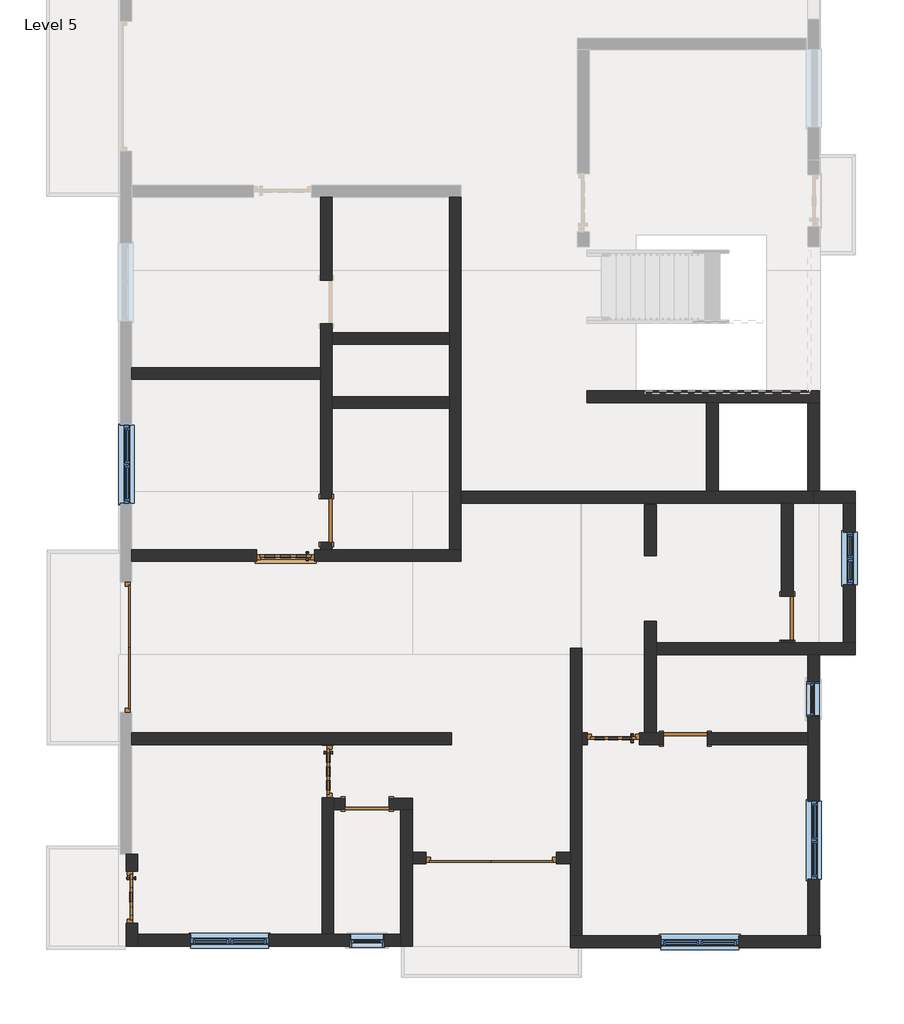
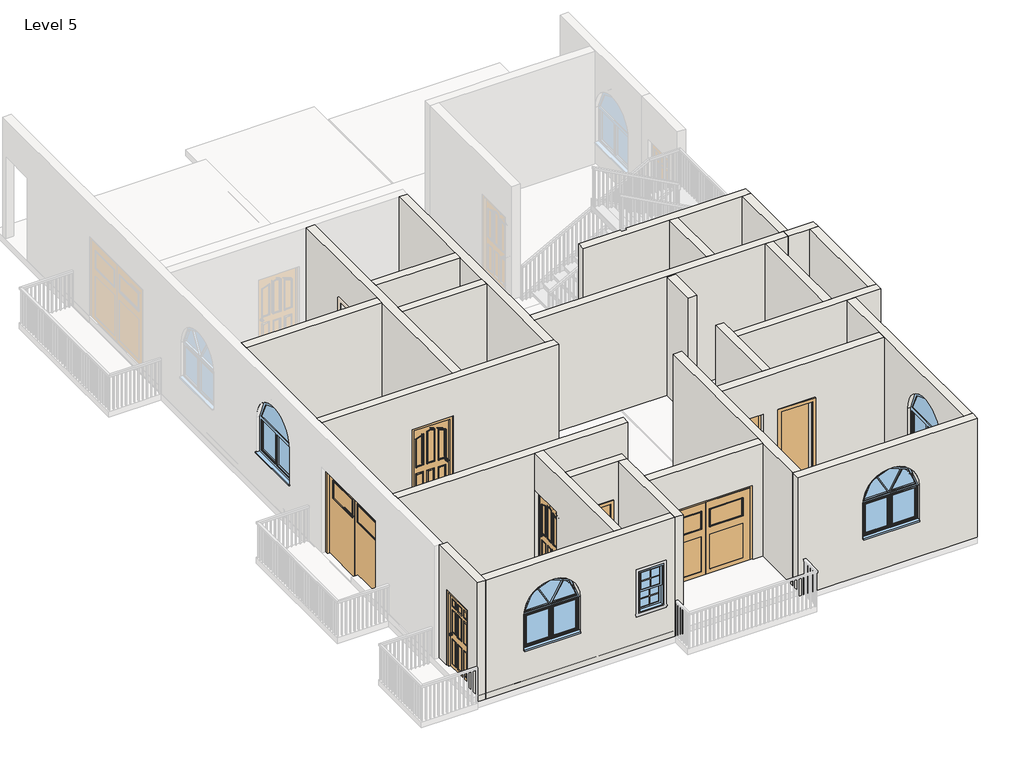
# One storey, part 1 of 7: 27 walls, 10 doors, 7 windows.
"""IFC4 building model written with IfcOpenShell, lengths in millimetres."""

from ifc_helpers import new_model, si_unit, frame, origin, place, context, project, spatial, polyline, circle_curve, outline, extrude, faceted_brep, transform, mapped, element, save
from ifc_brep_helpers import plane_surface, revolved_surface, advanced_brep
from components import doors_extsgl_5_910x2110mm_99758a98, doors_extsgl_6_1010x2110mm_b93c615f, doors_extsgl_6_1010x2110mm_efbaf1af, doors_extsgl_6_910x2110mm_72be2df1, doors_extsgl_6_910x2110mm_b26fcae4, doors_extsgl_6_910x2110mm_5dc58899, doors_extsgl_6_910x2110mm_16d7c084, doors_garage_timber_side_hung_glazing_2270x2050mm_ae99176d, doors_garage_timber_side_hung_glazing_2270x2200mm_badb7014, door_fadea3f2, door_53b1b562, window_679d2811, windows_arched_1360x910mm_c5754810, windows_dbl_w_glazing_bars_910x910mm_41eba874

model = new_model("IFC4")

# Units and contexts
model_context = context("Model", 3, world=origin())
ifc_project = project(units=[si_unit("LENGTHUNIT", "METRE", prefix="MILLI")], contexts=[model_context])

# Site, building, storey
site = spatial("IfcSite", under=ifc_project)
building = spatial("IfcBuilding", under=site)
storey = spatial("IfcBuildingStorey", under=building, Name="Level 5", Elevation=12192.0)

# Doors
placement = place(None, origin())
doors_extsgl_5_910x2110mm_shape = doors_extsgl_5_910x2110mm_99758a98(model_context)
element("IfcDoor", 1, ObjectType="Doors_ExtSgl_5 : 910x2110mm", at=placement, inside=storey, context=model_context, shape_type="MappedRepresentation", body=[
    mapped(doors_extsgl_5_910x2110mm_shape, transform((-6127.6013636, -9759.5108149, 12192.0), x_axis=(0.0, -1.0, 0.0), y_axis=(1.0, 0.0, 0.0), z_axis=(0.0, 0.0, 1.0))),
])
doors_extsgl_6_1010x2110mm_shape = doors_extsgl_6_1010x2110mm_b93c615f(model_context)
doors_extsgl_6_1010x2110mm_2_shape = doors_extsgl_6_1010x2110mm_efbaf1af(model_context)
element("IfcDoor", 2, ObjectType="Doors_ExtSgl_6 : 1010x2110mm", at=placement, inside=storey, context=model_context, shape_type="MappedRepresentation", body=[
    mapped(doors_extsgl_6_1010x2110mm_shape, transform((-3445.8775704, -3805.7037749, 12192.0), x_axis=(-1.0, 0.0, 0.0), y_axis=(0.0, -1.0, 0.0), z_axis=(0.0, 0.0, 1.0))),
    mapped(doors_extsgl_6_1010x2110mm_2_shape, transform((-3445.8775704, -3805.7037749, 12192.0), x_axis=(-1.0, 0.0, 0.0), y_axis=(0.0, -1.0, 0.0), z_axis=(0.0, 0.0, 1.0))),
])
doors_extsgl_6_910x2110mm_shape = doors_extsgl_6_910x2110mm_72be2df1(model_context)
doors_extsgl_6_910x2110mm_2_shape = doors_extsgl_6_910x2110mm_b26fcae4(model_context)
element("IfcDoor", 3, ObjectType="Doors_ExtSgl_6 : 910x2110mm", at=placement, inside=storey, context=model_context, shape_type="MappedRepresentation", body=[
    mapped(doors_extsgl_6_910x2110mm_shape, transform((2269.1224296, -6998.5466225, 12192.0), x_axis=(-1.0, 0.0, 0.0), y_axis=(0.0, -1.0, 0.0), z_axis=(0.0, 0.0, 1.0))),
    mapped(doors_extsgl_6_910x2110mm_2_shape, transform((2269.1224296, -6998.5466225, 12192.0), x_axis=(-1.0, 0.0, 0.0), y_axis=(0.0, -1.0, 0.0), z_axis=(0.0, 0.0, 1.0))),
])
doors_extsgl_6_910x2110mm_3_shape = doors_extsgl_6_910x2110mm_5dc58899(model_context)
doors_extsgl_6_910x2110mm_4_shape = doors_extsgl_6_910x2110mm_16d7c084(model_context)
element("IfcDoor", 4, ObjectType="Doors_ExtSgl_6 : 910x2110mm", at=placement, inside=storey, context=model_context, shape_type="MappedRepresentation", body=[
    mapped(doors_extsgl_6_910x2110mm_3_shape, transform((-2709.3109037, -7568.3747197, 12192.0), x_axis=(0.0, -1.0, 0.0), y_axis=(1.0, 0.0, 0.0), z_axis=(0.0, 0.0, 1.0))),
    mapped(doors_extsgl_6_910x2110mm_4_shape, transform((-2709.3109037, -7568.3747197, 12192.0), x_axis=(0.0, -1.0, 0.0), y_axis=(1.0, 0.0, 0.0), z_axis=(0.0, 0.0, 1.0))),
])
doors_garage_timber_side_hung_glazing_2270x2050mm_shape = doors_garage_timber_side_hung_glazing_2270x2050mm_ae99176d(model_context)
element("IfcDoor", 5, ObjectType="Doors_Garage_Timber_Side_Hung_Glazing : 2270x2050mm", at=placement, inside=storey, context=model_context, shape_type="MappedRepresentation", body=[
    mapped(doors_garage_timber_side_hung_glazing_2270x2050mm_shape, transform((141.8390963, -9078.0694836, 12192.0), x_axis=(-1.0, 0.0, 0.0), y_axis=(0.0, -1.0, 0.0), z_axis=(0.0, 0.0, 1.0))),
])
doors_garage_timber_side_hung_glazing_2270x2200mm_shape = doors_garage_timber_side_hung_glazing_2270x2200mm_badb7014(model_context)
element("IfcDoor", 6, ObjectType="Doors_Garage_Timber_Side_Hung_Glazing : 2270x2200mm", at=placement, inside=storey, context=model_context, shape_type="MappedRepresentation", body=[
    mapped(doors_garage_timber_side_hung_glazing_2270x2200mm_shape, transform((-6229.2013636, -5402.1251987, 12192.0), x_axis=(0.0, 1.0, 0.0), y_axis=(-1.0, 0.0, 0.0), z_axis=(0.0, 0.0, 1.0))),
])
door_shape = door_fadea3f2(model_context)
element("IfcDoor", 7, ObjectType="Single-Flush : 30\" x 80\"", at=placement, inside=storey, context=model_context, shape_type="MappedRepresentation", body=[
    mapped(door_shape, transform((-2023.5109037, -8138.2694836, 12192.0), x_axis=(-1.0, 0.0, 0.0), y_axis=(0.0, -1.0, 0.0), z_axis=(0.0, 0.0, 1.0))),
])
element("IfcDoor", 8, ObjectType="Single-Flush : 30\" x 80\"", at=placement, inside=storey, context=model_context, shape_type="MappedRepresentation", body=[
    mapped(door_shape, transform((5304.3890963, -4897.9037749, 12192.0), x_axis=(0.0, -1.0, 0.0), y_axis=(1.0, 0.0, 0.0), z_axis=(0.0, 0.0, 1.0))),
])
door_2_shape = door_53b1b562(model_context)
element("IfcDoor", 9, ObjectType="Single-Flush : 30\" x 80\"", at=placement, inside=storey, context=model_context, shape_type="MappedRepresentation", body=[
    mapped(door_2_shape, transform((-2734.7109037, -3196.1037749, 12192.0), x_axis=(0.0, 1.0, 0.0), y_axis=(-1.0, 0.0, 0.0), z_axis=(0.0, 0.0, 1.0))),
])
element("IfcDoor", 10, ObjectType="Single-Flush : 30\" x 80\"", at=placement, inside=storey, context=model_context, shape_type="MappedRepresentation", body=[
    mapped(door_2_shape, transform((3526.3890963, -6998.5466225, 12192.0), x_axis=(-1.0, 0.0, 0.0), y_axis=(0.0, -1.0, 0.0), z_axis=(0.0, 0.0, 1.0))),
])

# Walls
element("IfcWall", 11, ObjectType="Generic - 9\" w", at=placement, inside=storey, context=model_context, shape_type="Brep", body=[
    faceted_brep([(6485.4890963, -2688.1037749, 12192.0), (5863.1890963, -2688.1037749, 12192.0), (5761.5890963, -2688.1037749, 12192.0), (5761.5890963, -2688.1037749, 15240.0), (5863.1890963, -2688.1037749, 15240.0), (6485.4890963, -2688.1037749, 15240.0), (6485.4890963, -2891.3037749, 12192.0), (6485.4890963, -2891.3037749, 15240.0), (6282.2890963, -2891.3037749, 15240.0), (5761.5890963, -2891.3037749, 15240.0), (5761.5890963, -2891.3037749, 12192.0), (6282.2890963, -2891.3037749, 12192.0)], [[[0, 1, 2, 3, 4, 5]], [[6, 7, 8, 9, 10, 11]], [[2, 1, 0, 6, 11, 10]], [[3, 2, 10, 9]], [[5, 4, 3, 9, 8, 7]], [[0, 5, 7, 6]]]),
])
element("IfcWall", 12, ObjectType="Generic - 9\" w", at=placement, inside=storey, context=model_context, shape_type="Brep", body=[
    faceted_brep([(5761.5890963, -2688.1037749, 12192.0), (5659.9890963, -2688.1037749, 12192.0), (4097.8890963, -2688.1037749, 12192.0), (3894.6890963, -2688.1037749, 12192.0), (-385.2109037, -2688.1037749, 12192.0), (-385.2109037, -2688.1037749, 15240.0), (3894.6890963, -2688.1037749, 15240.0), (4097.8890963, -2688.1037749, 15240.0), (5659.9890963, -2688.1037749, 15240.0), (5761.5890963, -2688.1037749, 15240.0), (5761.5890963, -2891.3037749, 12192.0), (5761.5890963, -2891.3037749, 15240.0), (5405.9890963, -2891.3037749, 15240.0), (5202.7890963, -2891.3037749, 15240.0), (-385.2109037, -2891.3037749, 15240.0), (-385.2109037, -2891.3037749, 12192.0), (5202.7890963, -2891.3037749, 12192.0), (5405.9890963, -2891.3037749, 12192.0)], [[[0, 1, 2, 3, 4, 5, 6, 7, 8, 9]], [[10, 11, 12, 13, 14, 15, 16, 17]], [[4, 3, 2, 1, 0, 10, 17, 16, 15]], [[9, 8, 7, 6, 5, 14, 13, 12, 11]], [[0, 9, 11, 10]], [[5, 4, 15, 14]]]),
])
element("IfcWall", 13, ObjectType="Generic - 9\" w", at=placement, inside=storey, context=model_context, shape_type="SweptSolid", body=[
    extrude(outline(polyline([(3894.6890963, -2688.1037749), (3894.6890963, -1138.7037749), (4097.8890963, -1138.7037749), (4097.8890963, -2688.1037749), (3894.6890963, -2688.1037749)])), frame((0.0, 0.0, 12192.0), z_axis=(0.0, 0.0, 1.0), x_axis=(1.0, 0.0, 0.0)), (0.0, 0.0, 1.0), 3048.0),
])
element("IfcWall", 14, ObjectType="Generic - 9\" w", at=placement, inside=storey, context=model_context, shape_type="Brep", body=[
    faceted_brep([(5863.1890963, -935.5037749, 12192.0), (1812.4805171, -935.5037749, 12192.0), (1812.4805171, -935.5037749, 15240.0), (5863.1890963, -935.5037749, 15240.0), (5863.1890963, -1138.7037749, 12192.0), (5863.1890963, -1138.7037749, 15240.0), (5659.9890963, -1138.7037749, 15240.0), (4097.8890963, -1138.7037749, 15240.0), (3894.6890963, -1138.7037749, 15240.0), (1812.4805171, -1138.7037749, 15240.0), (1812.4805171, -1138.7037749, 12192.0), (3894.6890963, -1138.7037749, 12192.0), (4097.8890963, -1138.7037749, 12192.0), (5659.9890963, -1138.7037749, 12192.0)], [[[0, 1, 2, 3]], [[4, 5, 6, 7, 8, 9, 10, 11, 12, 13]], [[1, 0, 4, 13, 12, 11, 10]], [[2, 1, 10, 9]], [[3, 2, 9, 8, 7, 6, 5]], [[0, 3, 5, 4]]]),
])
element("IfcWall", 15, ObjectType="Generic - 9\" w", at=placement, inside=storey, context=model_context, shape_type="AdvancedBrep", body=[
    advanced_brep(
    [(1519.7890963, -10638.3037749, 12192.0), (5875.8890963, -10638.3037749, 12192.0), (5875.8890963, -10638.3037749, 15240.0), (1519.7890963, -10638.3037749, 15240.0), (4460.3890963, -10638.3037749, 13106.4), (3100.3890963, -10638.3037749, 13106.4), (3100.3890963, -10638.3037749, 14016.4), (4460.3890963, -10638.3037749, 14016.4), (1519.7890963, -10435.1037749, 12192.0), (1519.7890963, -10435.1037749, 15240.0), (1722.9890963, -10435.1037749, 15240.0), (5659.9890963, -10435.1037749, 15240.0), (5863.1890963, -10435.1037749, 15240.0), (5875.8890963, -10435.1037749, 15240.0), (5875.8890963, -10435.1037749, 12192.0), (5863.1890963, -10435.1037749, 12192.0), (5659.9890963, -10435.1037749, 12192.0), (1722.9890963, -10435.1037749, 12192.0), (4460.3890963, -10435.1037749, 13106.4), (4460.3890963, -10435.1037749, 14016.4), (3100.3890963, -10435.1037749, 14016.4), (3100.3890963, -10435.1037749, 13106.4)],
    [
        (0, 1),
        (1, 2),
        (2, 3),
        (3, 0),
        (4, 5),
        (5, 6),
        (6, 7, circle_curve(frame((3780.3890963, -10638.3037749, 14016.4), z_axis=(0.0, 1.0, 0.0), x_axis=(-1.0, 0.0, 0.0)), 680.0)),
        (7, 4),
        (8, 9),
        (9, 10),
        (10, 11),
        (11, 12),
        (12, 13),
        (13, 14),
        (14, 15),
        (15, 16),
        (16, 17),
        (17, 8),
        (18, 19),
        (19, 20, circle_curve(frame((3780.3890963, -10435.1037749, 14016.4), z_axis=(0.0, -1.0, 0.0), x_axis=(-1.0, 0.0, 0.0)), 680.0)),
        (20, 21),
        (21, 18),
        (0, 8),
        (14, 1),
        (13, 2),
        (9, 3),
        (18, 4),
        (7, 19),
        (6, 20),
        (5, 21),
    ],
    [
        plane_surface(frame((1722.9890963, -10638.3037749, 12192.0), z_axis=(0.0, -1.0, 0.0), x_axis=(1.0, 0.0, 0.0))),
        plane_surface(frame((1722.9890963, -10435.1037749, 12192.0), z_axis=(0.0, 1.0, 0.0), x_axis=(-1.0, 0.0, 0.0))),
        plane_surface(frame((1621.3890963, -10638.3037749, 12192.0), z_axis=(0.0, 0.0, -1.0), x_axis=(0.0, 1.0, 0.0))),
        plane_surface(frame((5875.8890963, -10638.3037749, 12192.0), z_axis=(1.0, 0.0, 0.0), x_axis=(0.0, 1.0, 0.0))),
        plane_surface(frame((5875.8890963, -10638.3037749, 15240.0), z_axis=(0.0, 0.0, 1.0), x_axis=(0.0, 1.0, 0.0))),
        plane_surface(frame((1519.7890963, -5418.6037749, 12192.0), z_axis=(-1.0, 0.0, 0.0), x_axis=(0.0, -1.0, 0.0))),
        plane_surface(frame((4460.3890963, -10435.1037749, 13106.4), z_axis=(-1.0, 0.0, 0.0), x_axis=(0.0, -1.0, 0.0))),
        revolved_surface(polyline([(3100.3890963, -10638.3037749, 14016.4), (3100.3890963, -10435.1037749, 14016.4)]), (3780.3890963, -10435.1037749, 14016.4), (0.0, -1.0, 0.0)),
        plane_surface(frame((3100.3890963, -10435.1037749, 14016.4), z_axis=(1.0, 0.0, 0.0), x_axis=(0.0, -1.0, 0.0))),
        plane_surface(frame((3100.3890963, -10435.1037749, 13106.4), z_axis=(0.0, 0.0, 1.0), x_axis=(0.0, -1.0, 0.0))),
    ],
    [
        (0, [[1, 2, 3, 4], [5, 6, 7, 8]]),
        (1, [[9, 10, 11, 12, 13, 14, 15, 16, 17, 18], [19, 20, 21, 22]]),
        (2, [[-1, 23, -18, -17, -16, -15, 24]]),
        (3, [[-2, -24, -14, 25]]),
        (4, [[-3, -25, -13, -12, -11, -10, 26]]),
        (5, [[-4, -26, -9, -23]]),
        (6, [[-19, 27, -8, 28]]),
        (7, [[-20, -28, -7, 29]]),
        (8, [[-21, -29, -6, 30]]),
        (9, [[-22, -30, -5, -27]]),
    ],
),
])
element("IfcWall", 16, ObjectType="Generic - 9\" w", at=placement, inside=storey, context=model_context, shape_type="AdvancedBrep", body=[
    advanced_brep(
    [(5863.1890963, -10435.1037749, 12192.0), (5863.1890963, -5532.9037749, 12192.0), (5863.1890963, -5532.9037749, 15240.0), (5863.1890963, -10435.1037749, 15240.0), (5863.1890963, -8087.6251987, 13106.4), (5863.1890963, -9447.6251987, 13106.4), (5863.1890963, -9447.6251987, 14016.4), (5863.1890963, -8087.6251987, 14016.4), (5863.1890963, -6618.7537749, 14173.2), (5863.1890963, -6009.1537749, 14173.2), (5863.1890963, -6009.1537749, 13106.4), (5863.1890963, -6618.7537749, 13106.4), (5659.9890963, -10435.1037749, 12192.0), (5659.9890963, -10435.1037749, 15240.0), (5659.9890963, -7100.1466225, 15240.0), (5659.9890963, -6896.9466225, 15240.0), (5659.9890963, -5532.9037749, 15240.0), (5659.9890963, -5532.9037749, 12192.0), (5659.9890963, -6896.9466225, 12192.0), (5659.9890963, -7100.1466225, 12192.0), (5659.9890963, -8087.6251987, 13106.4), (5659.9890963, -8087.6251987, 14016.4), (5659.9890963, -9447.6251987, 14016.4), (5659.9890963, -9447.6251987, 13106.4), (5659.9890963, -6618.7537749, 14173.2), (5659.9890963, -6618.7537749, 13106.4), (5659.9890963, -6009.1537749, 13106.4), (5659.9890963, -6009.1537749, 14173.2)],
    [
        (0, 1),
        (1, 2),
        (2, 3),
        (3, 0),
        (4, 5),
        (5, 6),
        (6, 7, circle_curve(frame((5863.1890963, -8767.6251987, 14016.4), z_axis=(-1.0, 0.0, 0.0), x_axis=(0.0, -1.0, 0.0)), 680.0)),
        (7, 4),
        (8, 9),
        (9, 10),
        (10, 11),
        (11, 8),
        (12, 13),
        (13, 14),
        (14, 15),
        (15, 16),
        (16, 17),
        (17, 18),
        (18, 19),
        (19, 12),
        (20, 21),
        (21, 22, circle_curve(frame((5659.9890963, -8767.6251987, 14016.4), z_axis=(1.0, 0.0, 0.0), x_axis=(0.0, -1.0, 0.0)), 680.0)),
        (22, 23),
        (23, 20),
        (24, 25),
        (25, 26),
        (26, 27),
        (27, 24),
        (0, 12),
        (17, 1),
        (2, 16),
        (13, 3),
        (20, 4),
        (7, 21),
        (6, 22),
        (5, 23),
        (24, 8),
        (11, 25),
        (10, 26),
        (9, 27),
    ],
    [
        plane_surface(frame((5863.1890963, -10435.1037749, 12192.0), z_axis=(1.0, 0.0, 0.0), x_axis=(0.0, 1.0, 0.0))),
        plane_surface(frame((5659.9890963, -10435.1037749, 12192.0), z_axis=(-1.0, 0.0, 0.0), x_axis=(0.0, -1.0, 0.0))),
        plane_surface(frame((5863.1890963, -10536.7037749, 12192.0), z_axis=(0.0, 0.0, -1.0), x_axis=(-1.0, 0.0, 0.0))),
        plane_surface(frame((5863.1890963, -5431.3037749, 15240.0), z_axis=(0.0, 0.0, 1.0), x_axis=(-1.0, 0.0, 0.0))),
        plane_surface(frame((1722.9890963, -10435.1037749, 12192.0), z_axis=(0.0, -1.0, 0.0), x_axis=(-1.0, 0.0, 0.0))),
        plane_surface(frame((3018.3890963, -5532.9037749, 12192.0), z_axis=(0.0, 1.0, 0.0), x_axis=(1.0, 0.0, 0.0))),
        plane_surface(frame((5659.9890963, -8087.6251987, 13106.4), z_axis=(0.0, -1.0, 0.0), x_axis=(1.0, 0.0, 0.0))),
        revolved_surface(polyline([(5863.1890963, -9447.6251987, 14016.4), (5659.9890963, -9447.6251987, 14016.4)]), (5659.9890963, -8767.6251987, 14016.4), (1.0, 0.0, 0.0)),
        plane_surface(frame((5659.9890963, -9447.6251987, 14016.4), z_axis=(0.0, 1.0, 0.0), x_axis=(1.0, 0.0, 0.0))),
        plane_surface(frame((5659.9890963, -9447.6251987, 13106.4), z_axis=(0.0, 0.0, 1.0), x_axis=(1.0, 0.0, 0.0))),
        plane_surface(frame((5659.9890963, -6618.7537749, 14173.2), z_axis=(0.0, 1.0, 0.0), x_axis=(1.0, 0.0, 0.0))),
        plane_surface(frame((5659.9890963, -6618.7537749, 13106.4), z_axis=(0.0, 0.0, 1.0), x_axis=(1.0, 0.0, 0.0))),
        plane_surface(frame((5659.9890963, -6009.1537749, 13106.4), z_axis=(0.0, -1.0, 0.0), x_axis=(1.0, 0.0, 0.0))),
        plane_surface(frame((5659.9890963, -6009.1537749, 14173.2), z_axis=(0.0, 0.0, -1.0), x_axis=(1.0, 0.0, 0.0))),
    ],
    [
        (0, [[1, 2, 3, 4], [5, 6, 7, 8], [9, 10, 11, 12]]),
        (1, [[13, 14, 15, 16, 17, 18, 19, 20], [21, 22, 23, 24], [25, 26, 27, 28]]),
        (2, [[-1, 29, -20, -19, -18, 30]]),
        (3, [[-3, 31, -16, -15, -14, 32]]),
        (4, [[-4, -32, -13, -29]]),
        (5, [[-2, -30, -17, -31]]),
        (6, [[-21, 33, -8, 34]]),
        (7, [[-22, -34, -7, 35]]),
        (8, [[-23, -35, -6, 36]]),
        (9, [[-24, -36, -5, -33]]),
        (10, [[-25, 37, -12, 38]]),
        (11, [[-26, -38, -11, 39]]),
        (12, [[-27, -39, -10, 40]]),
        (13, [[-28, -40, -9, -37]]),
    ],
),
])
element("IfcWall", 17, ObjectType="Generic - 9\" w", at=placement, inside=storey, context=model_context, shape_type="Brep", body=[
    faceted_brep([(5659.9890963, -1138.7037749, 12192.0), (5659.9890963, -2688.1037749, 12192.0), (5659.9890963, -2688.1037749, 15240.0), (5659.9890963, -1138.7037749, 15240.0), (5863.1890963, -1138.7037749, 12192.0), (5863.1890963, -1138.7037749, 15240.0), (5863.1890963, -2688.1037749, 15240.0), (5863.1890963, -2688.1037749, 12192.0), (5761.5890963, -2688.1037749, 12192.0), (5761.5890963, -2688.1037749, 15240.0)], [[[0, 1, 2, 3]], [[4, 5, 6, 7]], [[1, 0, 4, 7, 8]], [[3, 2, 9, 6, 5]], [[2, 1, 8, 7, 6, 9]], [[0, 3, 5, 4]]]),
])
element("IfcWall", 18, ObjectType="Generic - 9\" w", at=placement, inside=storey, context=model_context, shape_type="Brep", body=[
    faceted_brep([(-6229.2013636, -10214.5441482, 14302.0), (-6229.2013636, -10214.5441482, 12192.0), (-6229.2013636, -10612.9037749, 12192.0), (-6229.2013636, -10612.9037749, 15240.0), (-6229.2013636, -9007.7845215, 15240.0), (-6229.2013636, -9007.7845215, 12192.0), (-6229.2013636, -9304.5441482, 12192.0), (-6229.2013636, -9304.5441482, 14302.0), (-6026.0013636, -10612.9037749, 12192.0), (-6026.0013636, -10409.7037749, 12192.0), (-6026.0013636, -10214.5441482, 12192.0), (-6026.0013636, -10214.5441482, 14302.0), (-6026.0013636, -9304.5441482, 14302.0), (-6026.0013636, -9304.5441482, 12192.0), (-6026.0013636, -9007.7845215, 12192.0), (-6026.0013636, -9007.7845215, 15240.0), (-6026.0013636, -10409.7037749, 15240.0), (-6026.0013636, -10612.9037749, 15240.0), (-6127.6013636, -9007.7845215, 12192.0), (-6127.6013636, -9007.7845215, 15240.0)], [[[0, 1, 2, 3, 4, 5, 6, 7]], [[8, 9, 10, 11, 12, 13, 14, 15, 16, 17]], [[6, 5, 18, 14, 13]], [[2, 1, 10, 9, 8]], [[4, 3, 17, 16, 15, 19]], [[5, 4, 19, 15, 14, 18]], [[13, 12, 7, 6]], [[11, 10, 1, 0]], [[12, 11, 0, 7]], [[3, 2, 8, 17]]]),
])
element("IfcWall", 19, ObjectType="Generic - 9\" w", at=placement, inside=storey, context=model_context, shape_type="AdvancedBrep", body=[
    advanced_brep(
    [(-6026.0013636, -10612.9037749, 12192.0), (-1439.3109037, -10612.9037749, 12192.0), (-1439.3109037, -10612.9037749, 15240.0), (-6026.0013636, -10612.9037749, 15240.0), (-3738.4561337, -10612.9037749, 13106.4), (-5098.4561337, -10612.9037749, 13106.4), (-5098.4561337, -10612.9037749, 14016.4), (-3738.4561337, -10612.9037749, 14016.4), (-1718.7109037, -10612.9037749, 14173.2), (-1718.7109037, -10612.9037749, 13106.4), (-2328.3109037, -10612.9037749, 13106.4), (-2328.3109037, -10612.9037749, 14173.2), (-6026.0013636, -10409.7037749, 12192.0), (-6026.0013636, -10409.7037749, 15240.0), (-2810.9109037, -10409.7037749, 15240.0), (-2607.7109037, -10409.7037749, 15240.0), (-1439.3109037, -10409.7037749, 15240.0), (-1439.3109037, -10409.7037749, 12192.0), (-2607.7109037, -10409.7037749, 12192.0), (-2810.9109037, -10409.7037749, 12192.0), (-3738.4561337, -10409.7037749, 13106.4), (-3738.4561337, -10409.7037749, 14016.4), (-5098.4561337, -10409.7037749, 14016.4), (-5098.4561337, -10409.7037749, 13106.4), (-1718.7109037, -10409.7037749, 14173.2), (-2328.3109037, -10409.7037749, 14173.2), (-2328.3109037, -10409.7037749, 13106.4), (-1718.7109037, -10409.7037749, 13106.4)],
    [
        (0, 1),
        (1, 2),
        (2, 3),
        (3, 0),
        (4, 5),
        (5, 6),
        (6, 7, circle_curve(frame((-4418.4561337, -10612.9037749, 14016.4), z_axis=(0.0, 1.0, 0.0), x_axis=(-1.0, 0.0, 0.0)), 680.0)),
        (7, 4),
        (8, 9),
        (9, 10),
        (10, 11),
        (11, 8),
        (12, 13),
        (13, 14),
        (14, 15),
        (15, 16),
        (16, 17),
        (17, 18),
        (18, 19),
        (19, 12),
        (20, 21),
        (21, 22, circle_curve(frame((-4418.4561337, -10409.7037749, 14016.4), z_axis=(0.0, -1.0, 0.0), x_axis=(-1.0, 0.0, 0.0)), 680.0)),
        (22, 23),
        (23, 20),
        (24, 25),
        (25, 26),
        (26, 27),
        (27, 24),
        (0, 12),
        (17, 1),
        (2, 16),
        (13, 3),
        (20, 4),
        (7, 21),
        (6, 22),
        (5, 23),
        (8, 24),
        (27, 9),
        (26, 10),
        (25, 11),
    ],
    [
        plane_surface(frame((-6229.2013636, -10612.9037749, 12192.0), z_axis=(0.0, -1.0, 0.0), x_axis=(1.0, 0.0, 0.0))),
        plane_surface(frame((-6229.2013636, -10409.7037749, 12192.0), z_axis=(0.0, 1.0, 0.0), x_axis=(-1.0, 0.0, 0.0))),
        plane_surface(frame((-6127.6013636, -10612.9037749, 12192.0), z_axis=(0.0, 0.0, -1.0), x_axis=(0.0, 1.0, 0.0))),
        plane_surface(frame((-1337.7109037, -10612.9037749, 15240.0), z_axis=(0.0, 0.0, 1.0), x_axis=(0.0, 1.0, 0.0))),
        plane_surface(frame((-1439.3109037, -8239.8694836, 12192.0), z_axis=(1.0, 0.0, 0.0), x_axis=(0.0, -1.0, 0.0))),
        plane_surface(frame((-6026.0013636, -9109.3845215, 12192.0), z_axis=(-1.0, 0.0, 0.0), x_axis=(0.0, 1.0, 0.0))),
        plane_surface(frame((-3738.4561337, -10409.7037749, 13106.4), z_axis=(-1.0, 0.0, 0.0), x_axis=(0.0, -1.0, 0.0))),
        revolved_surface(polyline([(-5098.4561337, -10612.9037749, 14016.4), (-5098.4561337, -10409.7037749, 14016.4)]), (-4418.4561337, -10409.7037749, 14016.4), (0.0, -1.0, 0.0)),
        plane_surface(frame((-5098.4561337, -10409.7037749, 14016.4), z_axis=(1.0, 0.0, 0.0), x_axis=(0.0, -1.0, 0.0))),
        plane_surface(frame((-5098.4561337, -10409.7037749, 13106.4), z_axis=(0.0, 0.0, 1.0), x_axis=(0.0, -1.0, 0.0))),
        plane_surface(frame((-1718.7109037, -10612.9037749, 14173.2), z_axis=(-1.0, 0.0, 0.0), x_axis=(0.0, 1.0, 0.0))),
        plane_surface(frame((-1718.7109037, -10612.9037749, 13106.4), z_axis=(0.0, 0.0, 1.0), x_axis=(0.0, 1.0, 0.0))),
        plane_surface(frame((-2328.3109037, -10612.9037749, 13106.4), z_axis=(1.0, 0.0, 0.0), x_axis=(0.0, 1.0, 0.0))),
        plane_surface(frame((-2328.3109037, -10612.9037749, 14173.2), z_axis=(0.0, 0.0, -1.0), x_axis=(0.0, 1.0, 0.0))),
    ],
    [
        (0, [[1, 2, 3, 4], [5, 6, 7, 8], [9, 10, 11, 12]]),
        (1, [[13, 14, 15, 16, 17, 18, 19, 20], [21, 22, 23, 24], [25, 26, 27, 28]]),
        (2, [[-1, 29, -20, -19, -18, 30]]),
        (3, [[-3, 31, -16, -15, -14, 32]]),
        (4, [[-2, -30, -17, -31]]),
        (5, [[-4, -32, -13, -29]]),
        (6, [[-21, 33, -8, 34]]),
        (7, [[-22, -34, -7, 35]]),
        (8, [[-23, -35, -6, 36]]),
        (9, [[-24, -36, -5, -33]]),
        (10, [[-9, 37, -28, 38]]),
        (11, [[-10, -38, -27, 39]]),
        (12, [[-11, -39, -26, 40]]),
        (13, [[-12, -40, -25, -37]]),
    ],
),
])
element("IfcWall", 20, ObjectType="Generic -4.5\" p", at=placement, inside=storey, context=model_context, shape_type="Brep", body=[
    faceted_brep([(-2836.3109037, 232.8962251, 12192.0), (-2836.3109037, -529.1037749, 12192.0), (-2836.3109037, -732.3037749, 12192.0), (-2836.3109037, -2815.1037749, 12192.0), (-2836.3109037, -2815.1037749, 14224.0), (-2836.3109037, -3577.1037749, 14224.0), (-2836.3109037, -3577.1037749, 12192.0), (-2836.3109037, -3704.1037749, 12192.0), (-2836.3109037, -3704.1037749, 15240.0), (-2836.3109037, -732.3037749, 15240.0), (-2836.3109037, -529.1037749, 15240.0), (-2836.3109037, 2442.6962251, 15240.0), (-2836.3109037, 2442.6962251, 12192.0), (-2836.3109037, 994.8962251, 12192.0), (-2836.3109037, 994.8962251, 14224.0), (-2836.3109037, 232.8962251, 14224.0), (-2633.1109037, -2815.1037749, 14224.0), (-2633.1109037, -2815.1037749, 12192.0), (-2633.1109037, -1240.3037749, 12192.0), (-2633.1109037, -1037.1037749, 12192.0), (-2633.1109037, -122.7037749, 12192.0), (-2633.1109037, 80.4962251, 12192.0), (-2633.1109037, 232.8962251, 12192.0), (-2633.1109037, 232.8962251, 14224.0), (-2633.1109037, 994.8962251, 14224.0), (-2633.1109037, 994.8962251, 12192.0), (-2633.1109037, 2442.6962251, 12192.0), (-2633.1109037, 2442.6962251, 15240.0), (-2633.1109037, 80.4962251, 15240.0), (-2633.1109037, -122.7037749, 15240.0), (-2633.1109037, -1037.1037749, 15240.0), (-2633.1109037, -1240.3037749, 15240.0), (-2633.1109037, -3704.1037749, 15240.0), (-2633.1109037, -3704.1037749, 12192.0), (-2633.1109037, -3577.1037749, 12192.0), (-2633.1109037, -3577.1037749, 14224.0)], [[[0, 1, 2, 3, 4, 5, 6, 7, 8, 9, 10, 11, 12, 13, 14, 15]], [[16, 17, 18, 19, 20, 21, 22, 23, 24, 25, 26, 27, 28, 29, 30, 31, 32, 33, 34, 35]], [[26, 25, 13, 12]], [[34, 33, 7, 6]], [[22, 21, 20, 19, 18, 17, 3, 2, 1, 0]], [[11, 10, 9, 8, 32, 31, 30, 29, 28, 27]], [[12, 11, 27, 26]], [[8, 7, 33, 32]], [[14, 13, 25, 24]], [[15, 14, 24, 23]], [[0, 15, 23, 22]], [[4, 3, 17, 16]], [[5, 4, 16, 35]], [[6, 5, 35, 34]]]),
])
element("IfcWall", 21, ObjectType="Generic -4.5\" p", at=placement, inside=storey, context=model_context, shape_type="Brep", body=[
    faceted_brep([(-6127.6013636, -3907.3037749, 12192.0), (-3950.9109037, -3907.3037749, 12192.0), (-3950.9109037, -3907.3037749, 14302.0), (-2940.9109037, -3907.3037749, 14302.0), (-2940.9109037, -3907.3037749, 12192.0), (-385.2109037, -3907.3037749, 12192.0), (-385.2109037, -3907.3037749, 15240.0), (-6127.6013636, -3907.3037749, 15240.0), (-3950.9109037, -3704.1037749, 14302.0), (-3950.9109037, -3704.1037749, 12192.0), (-6127.6013636, -3704.1037749, 12192.0), (-6127.6013636, -3704.1037749, 15240.0), (-2836.3109037, -3704.1037749, 15240.0), (-2633.1109037, -3704.1037749, 15240.0), (-588.4109037, -3704.1037749, 15240.0), (-385.2109037, -3704.1037749, 15240.0), (-385.2109037, -3704.1037749, 12192.0), (-588.4109037, -3704.1037749, 12192.0), (-2633.1109037, -3704.1037749, 12192.0), (-2836.3109037, -3704.1037749, 12192.0), (-2940.9109037, -3704.1037749, 12192.0), (-2940.9109037, -3704.1037749, 14302.0)], [[[0, 1, 2, 3, 4, 5, 6, 7]], [[8, 9, 10, 11, 12, 13, 14, 15, 16, 17, 18, 19, 20, 21]], [[10, 9, 1, 0]], [[20, 19, 18, 17, 16, 5, 4]], [[7, 6, 15, 14, 13, 12, 11]], [[6, 5, 16, 15]], [[4, 3, 21, 20]], [[2, 1, 9, 8]], [[3, 2, 8, 21]], [[0, 7, 11, 10]]]),
])
element("IfcWall", 22, ObjectType="Generic -4.5\" p", at=placement, inside=storey, context=model_context, shape_type="Brep", body=[
    faceted_brep([(-385.2109037, -3704.1037749, 12192.0), (-385.2109037, -2891.3037749, 12192.0), (-385.2109037, -2688.1037749, 12192.0), (-385.2109037, 2442.6962251, 12192.0), (-385.2109037, 2442.6962251, 15240.0), (-385.2109037, -2688.1037749, 15240.0), (-385.2109037, -2891.3037749, 15240.0), (-385.2109037, -3704.1037749, 15240.0), (-588.4109037, -3704.1037749, 12192.0), (-588.4109037, -3704.1037749, 15240.0), (-588.4109037, -1240.3037749, 15240.0), (-588.4109037, -1037.1037749, 15240.0), (-588.4109037, -122.7037749, 15240.0), (-588.4109037, 80.4962251, 15240.0), (-588.4109037, 2442.6962251, 15240.0), (-588.4109037, 2442.6962251, 12192.0), (-588.4109037, 80.4962251, 12192.0), (-588.4109037, -122.7037749, 12192.0), (-588.4109037, -1037.1037749, 12192.0), (-588.4109037, -1240.3037749, 12192.0)], [[[0, 1, 2, 3, 4, 5, 6, 7]], [[8, 9, 10, 11, 12, 13, 14, 15, 16, 17, 18, 19]], [[3, 2, 1, 0, 8, 19, 18, 17, 16, 15]], [[7, 6, 5, 4, 14, 13, 12, 11, 10, 9]], [[4, 3, 15, 14]], [[0, 7, 9, 8]]]),
])
element("IfcWall", 23, ObjectType="Generic -4.5\" p", at=placement, inside=storey, context=model_context, shape_type="SweptSolid", body=[
    extrude(outline(polyline([(-588.4109037, -122.7037749), (-2633.1109037, -122.7037749), (-2633.1109037, 80.4962251), (-588.4109037, 80.4962251), (-588.4109037, -122.7037749)])), frame((0.0, 0.0, 12192.0), z_axis=(0.0, 0.0, 1.0), x_axis=(1.0, 0.0, 0.0)), (0.0, 0.0, 1.0), 3048.0),
])
element("IfcWall", 24, ObjectType="Generic -4.5\" p", at=placement, inside=storey, context=model_context, shape_type="SweptSolid", body=[
    extrude(outline(polyline([(-2836.3109037, -732.3037749), (-6127.6013636, -732.3037749), (-6127.6013636, -529.1037749), (-2836.3109037, -529.1037749), (-2836.3109037, -732.3037749)])), frame((0.0, 0.0, 12192.0), z_axis=(0.0, 0.0, 1.0), x_axis=(1.0, 0.0, 0.0)), (0.0, 0.0, 1.0), 3048.0),
])
element("IfcWall", 25, ObjectType="Generic -4.5\" p", at=placement, inside=storey, context=model_context, shape_type="SweptSolid", body=[
    extrude(outline(polyline([(-588.4109037, -1240.3037749), (-2633.1109037, -1240.3037749), (-2633.1109037, -1037.1037749), (-588.4109037, -1037.1037749), (-588.4109037, -1240.3037749)])), frame((0.0, 0.0, 12192.0), z_axis=(0.0, 0.0, 1.0), x_axis=(1.0, 0.0, 0.0)), (0.0, 0.0, 1.0), 3048.0),
])
element("IfcWall", 26, ObjectType="Generic -4.5\" p", at=placement, inside=storey, context=model_context, shape_type="Brep", body=[
    faceted_brep([(-6127.6013636, -7100.1466225, 12192.0), (-2810.9109037, -7100.1466225, 12192.0), (-2607.7109037, -7100.1466225, 12192.0), (-550.3109037, -7100.1466225, 12192.0), (-550.3109037, -7100.1466225, 15240.0), (-2607.7109037, -7100.1466225, 15240.0), (-2810.9109037, -7100.1466225, 15240.0), (-6127.6013636, -7100.1466225, 15240.0), (-6127.6013636, -6896.9466225, 12192.0), (-6127.6013636, -6896.9466225, 15240.0), (-550.3109037, -6896.9466225, 15240.0), (-550.3109037, -6896.9466225, 12192.0)], [[[0, 1, 2, 3, 4, 5, 6, 7]], [[8, 9, 10, 11]], [[3, 2, 1, 0, 8, 11]], [[4, 3, 11, 10]], [[7, 6, 5, 4, 10, 9]], [[0, 7, 9, 8]]]),
])
element("IfcWall", 27, ObjectType="Generic -4.5\" p", at=placement, inside=storey, context=model_context, shape_type="Brep", body=[
    faceted_brep([(-2607.7109037, -10409.7037749, 12192.0), (-2607.7109037, -8239.8694836, 12192.0), (-2607.7109037, -8036.6694836, 12192.0), (-2607.7109037, -8023.4080531, 12192.0), (-2607.7109037, -8023.4080531, 14302.0), (-2607.7109037, -7113.4080531, 14302.0), (-2607.7109037, -7113.4080531, 12192.0), (-2607.7109037, -7100.1466225, 12192.0), (-2607.7109037, -7100.1466225, 15240.0), (-2607.7109037, -8036.6694836, 15240.0), (-2607.7109037, -8239.8694836, 15240.0), (-2607.7109037, -10409.7037749, 15240.0), (-2810.9109037, -8023.4080531, 14302.0), (-2810.9109037, -8023.4080531, 12192.0), (-2810.9109037, -10409.7037749, 12192.0), (-2810.9109037, -10409.7037749, 15240.0), (-2810.9109037, -7100.1466225, 15240.0), (-2810.9109037, -7100.1466225, 12192.0), (-2810.9109037, -7113.4080531, 12192.0), (-2810.9109037, -7113.4080531, 14302.0)], [[[0, 1, 2, 3, 4, 5, 6, 7, 8, 9, 10, 11]], [[12, 13, 14, 15, 16, 17, 18, 19]], [[18, 17, 7, 6]], [[14, 13, 3, 2, 1, 0]], [[11, 10, 9, 8, 16, 15]], [[8, 7, 17, 16]], [[6, 5, 19, 18]], [[4, 3, 13, 12]], [[5, 4, 12, 19]], [[0, 11, 15, 14]]]),
])
element("IfcWall", 28, ObjectType="Generic -4.5\" p", at=placement, inside=storey, context=model_context, shape_type="Brep", body=[
    faceted_brep([(-2607.7109037, -8239.8694836, 12192.0), (-2404.5109037, -8239.8694836, 12192.0), (-2404.5109037, -8239.8694836, 14224.0), (-1642.5109037, -8239.8694836, 14224.0), (-1642.5109037, -8239.8694836, 12192.0), (-1439.3109037, -8239.8694836, 12192.0), (-1236.1109037, -8239.8694836, 12192.0), (-1236.1109037, -8239.8694836, 15240.0), (-1439.3109037, -8239.8694836, 15240.0), (-2607.7109037, -8239.8694836, 15240.0), (-2404.5109037, -8036.6694836, 14224.0), (-2404.5109037, -8036.6694836, 12192.0), (-2607.7109037, -8036.6694836, 12192.0), (-2607.7109037, -8036.6694836, 15240.0), (-1236.1109037, -8036.6694836, 15240.0), (-1236.1109037, -8036.6694836, 12192.0), (-1642.5109037, -8036.6694836, 12192.0), (-1642.5109037, -8036.6694836, 14224.0)], [[[0, 1, 2, 3, 4, 5, 6, 7, 8, 9]], [[10, 11, 12, 13, 14, 15, 16, 17]], [[16, 15, 6, 5, 4]], [[12, 11, 1, 0]], [[9, 8, 7, 14, 13]], [[0, 9, 13, 12]], [[7, 6, 15, 14]], [[2, 1, 11, 10]], [[3, 2, 10, 17]], [[4, 3, 17, 16]]]),
])
element("IfcWall", 29, ObjectType="Generic -4.5\" p", at=placement, inside=storey, context=model_context, shape_type="Brep", body=[
    faceted_brep([(-1439.3109037, -8239.8694836, 12192.0), (-1439.3109037, -10409.7037749, 12192.0), (-1439.3109037, -10612.9037749, 12192.0), (-1439.3109037, -10612.9037749, 15240.0), (-1439.3109037, -10409.7037749, 15240.0), (-1439.3109037, -8239.8694836, 15240.0), (-1236.1109037, -8239.8694836, 12192.0), (-1236.1109037, -8239.8694836, 15240.0), (-1236.1109037, -8976.4694836, 15240.0), (-1236.1109037, -9179.6694836, 15240.0), (-1236.1109037, -10612.9037749, 15240.0), (-1236.1109037, -10612.9037749, 12192.0), (-1236.1109037, -9179.6694836, 12192.0), (-1236.1109037, -8976.4694836, 12192.0)], [[[0, 1, 2, 3, 4, 5]], [[6, 7, 8, 9, 10, 11, 12, 13]], [[2, 1, 0, 6, 13, 12, 11]], [[5, 4, 3, 10, 9, 8, 7]], [[3, 2, 11, 10]], [[0, 5, 7, 6]]]),
])
element("IfcWall", 30, ObjectType="Generic -4.5\" p", at=placement, inside=storey, context=model_context, shape_type="SweptSolid", body=[
    extrude(outline(polyline([(12192.0, -1236.1109037), (12192.0, -993.1609037), (14242.0, -993.1609037), (14242.0, 1276.8390963), (12192.0, 1276.8390963), (12192.0, 1519.7890963), (15240.0, 1519.7890963), (15240.0, -1236.1109037), (12192.0, -1236.1109037)])), frame((0.0, -9179.6694836, 0.0), z_axis=(0.0, 1.0, 0.0), x_axis=(0.0, 0.0, 1.0)), (0.0, 0.0, 1.0), 203.2),
])
element("IfcWall", 31, ObjectType="Generic -4.5\" p", at=placement, inside=storey, context=model_context, shape_type="Brep", body=[
    faceted_brep([(1519.7890963, -5418.6037749, 12192.0), (1519.7890963, -8976.4694836, 12192.0), (1519.7890963, -9179.6694836, 12192.0), (1519.7890963, -10435.1037749, 12192.0), (1519.7890963, -10435.1037749, 15240.0), (1519.7890963, -9179.6694836, 15240.0), (1519.7890963, -8976.4694836, 15240.0), (1519.7890963, -5418.6037749, 15240.0), (1722.9890963, -5418.6037749, 12192.0), (1722.9890963, -5418.6037749, 15240.0), (1722.9890963, -6896.9466225, 15240.0), (1722.9890963, -7100.1466225, 15240.0), (1722.9890963, -10435.1037749, 15240.0), (1722.9890963, -10435.1037749, 12192.0), (1722.9890963, -7100.1466225, 12192.0), (1722.9890963, -6896.9466225, 12192.0)], [[[0, 1, 2, 3, 4, 5, 6, 7]], [[8, 9, 10, 11, 12, 13, 14, 15]], [[3, 2, 1, 0, 8, 15, 14, 13]], [[7, 6, 5, 4, 12, 11, 10, 9]], [[0, 7, 9, 8]], [[4, 3, 13, 12]]]),
])
element("IfcWall", 32, ObjectType="Generic -4.5\" p", at=placement, inside=storey, context=model_context, shape_type="Brep", body=[
    faceted_brep([(2724.0890963, -7100.1466225, 12192.0), (3145.3890963, -7100.1466225, 12192.0), (3145.3890963, -7100.1466225, 14224.0), (3907.3890963, -7100.1466225, 14224.0), (3907.3890963, -7100.1466225, 12192.0), (5659.9890963, -7100.1466225, 12192.0), (5659.9890963, -7100.1466225, 15240.0), (1722.9890963, -7100.1466225, 15240.0), (1722.9890963, -7100.1466225, 12192.0), (1814.0890963, -7100.1466225, 12192.0), (1814.0890963, -7100.1466225, 14302.0), (2724.0890963, -7100.1466225, 14302.0), (3145.3890963, -6896.9466225, 14224.0), (3145.3890963, -6896.9466225, 12192.0), (3018.3890963, -6896.9466225, 12192.0), (2815.1890963, -6896.9466225, 12192.0), (2724.0890963, -6896.9466225, 12192.0), (2724.0890963, -6896.9466225, 14302.0), (1814.0890963, -6896.9466225, 14302.0), (1814.0890963, -6896.9466225, 12192.0), (1722.9890963, -6896.9466225, 12192.0), (1722.9890963, -6896.9466225, 15240.0), (2815.1890963, -6896.9466225, 15240.0), (3018.3890963, -6896.9466225, 15240.0), (5659.9890963, -6896.9466225, 15240.0), (5659.9890963, -6896.9466225, 12192.0), (3907.3890963, -6896.9466225, 12192.0), (3907.3890963, -6896.9466225, 14224.0)], [[[0, 1, 2, 3, 4, 5, 6, 7, 8, 9, 10, 11]], [[12, 13, 14, 15, 16, 17, 18, 19, 20, 21, 22, 23, 24, 25, 26, 27]], [[20, 19, 9, 8]], [[26, 25, 5, 4]], [[16, 15, 14, 13, 1, 0]], [[7, 6, 24, 23, 22, 21]], [[6, 5, 25, 24]], [[8, 7, 21, 20]], [[0, 11, 17, 16]], [[10, 9, 19, 18]], [[11, 10, 18, 17]], [[2, 1, 13, 12]], [[3, 2, 12, 27]], [[4, 3, 27, 26]]]),
])
element("IfcWall", 33, ObjectType="Generic -4.5\" p", at=placement, inside=storey, context=model_context, shape_type="Brep", body=[
    faceted_brep([(3018.3890963, -6896.9466225, 12192.0), (3018.3890963, -5532.9037749, 12192.0), (3018.3890963, -5329.7037749, 12192.0), (3018.3890963, -4949.7445151, 12192.0), (3018.3890963, -4949.7445151, 15240.0), (3018.3890963, -5329.7037749, 15240.0), (3018.3890963, -5532.9037749, 15240.0), (3018.3890963, -6896.9466225, 15240.0), (2815.1890963, -6896.9466225, 12192.0), (2815.1890963, -6896.9466225, 15240.0), (2815.1890963, -4949.7445151, 15240.0), (2815.1890963, -4949.7445151, 12192.0)], [[[0, 1, 2, 3, 4, 5, 6, 7]], [[8, 9, 10, 11]], [[3, 2, 1, 0, 8, 11]], [[4, 3, 11, 10]], [[7, 6, 5, 4, 10, 9]], [[0, 7, 9, 8]]]),
])
element("IfcWall", 34, ObjectType="Generic -4.5\" p", at=placement, inside=storey, context=model_context, shape_type="Brep", body=[
    faceted_brep([(3018.3890963, -5532.9037749, 12192.0), (5659.9890963, -5532.9037749, 12192.0), (5863.1890963, -5532.9037749, 12192.0), (6485.4890963, -5532.9037749, 12192.0), (6485.4890963, -5532.9037749, 15240.0), (5863.1890963, -5532.9037749, 15240.0), (5659.9890963, -5532.9037749, 15240.0), (3018.3890963, -5532.9037749, 15240.0), (3018.3890963, -5329.7037749, 12192.0), (3018.3890963, -5329.7037749, 15240.0), (5202.7890963, -5329.7037749, 15240.0), (5405.9890963, -5329.7037749, 15240.0), (6282.2890963, -5329.7037749, 15240.0), (6485.4890963, -5329.7037749, 15240.0), (6485.4890963, -5329.7037749, 12192.0), (6282.2890963, -5329.7037749, 12192.0), (5405.9890963, -5329.7037749, 12192.0), (5202.7890963, -5329.7037749, 12192.0)], [[[0, 1, 2, 3, 4, 5, 6, 7]], [[8, 9, 10, 11, 12, 13, 14, 15, 16, 17]], [[3, 2, 1, 0, 8, 17, 16, 15, 14]], [[7, 6, 5, 4, 13, 12, 11, 10, 9]], [[0, 7, 9, 8]], [[4, 3, 14, 13]]]),
])
element("IfcWall", 35, ObjectType="Generic -4.5\" p", at=placement, inside=storey, context=model_context, shape_type="SweptSolid", body=[
    extrude(outline(polyline([(-5329.7037749, 12192.0), (-5329.7037749, 15240.0), (-2891.3037749, 15240.0), (-2891.3037749, 12192.0), (-5329.7037749, 12192.0)]), holes=[polyline([(-3401.5037749, 14016.4), (-4311.5037749, 14016.4), (-4311.5037749, 13106.4), (-3401.5037749, 13106.4), (-3401.5037749, 14016.4)])]), frame((6282.2890963, 0.0, 0.0), z_axis=(1.0, 0.0, 0.0), x_axis=(0.0, 1.0, 0.0)), (0.0, 0.0, 1.0), 203.2),
])
element("IfcWall", 36, ObjectType="Generic -4.5\" p", at=placement, inside=storey, context=model_context, shape_type="SweptSolid", body=[
    extrude(outline(polyline([(-5278.9037749, 14224.0), (-5278.9037749, 12192.0), (-5329.7037749, 12192.0), (-5329.7037749, 15240.0), (-2891.3037749, 15240.0), (-2891.3037749, 12192.0), (-4516.9037749, 12192.0), (-4516.9037749, 14224.0), (-5278.9037749, 14224.0)])), frame((5202.7890963, 0.0, 0.0), z_axis=(1.0, 0.0, 0.0), x_axis=(0.0, 1.0, 0.0)), (0.0, 0.0, 1.0), 203.2),
])
element("IfcWall", 37, ObjectType="Generic -4.5\" p", at=placement, inside=storey, context=model_context, shape_type="SweptSolid", body=[
    extrude(outline(polyline([(2815.1890963, -3808.4464026), (2815.1890963, -2916.7037749), (3018.3890963, -2916.7037749), (3018.3890963, -3808.4464026), (2815.1890963, -3808.4464026)])), frame((0.0, 0.0, 12192.0), z_axis=(0.0, 0.0, 1.0), x_axis=(1.0, 0.0, 0.0)), (0.0, 0.0, 1.0), 3048.0),
])

# Windows
window_shape = window_679d2811(model_context)
element("IfcWindow", 38, ObjectType="Window-Double-Hung : 24\" x 42\"", at=placement, inside=storey, context=model_context, shape_type="MappedRepresentation", body=[
    mapped(window_shape, transform((5761.5890963, -6313.9537749, 12192.0), x_axis=(0.0, 1.0, 0.0), y_axis=(-1.0, 0.0, 0.0), z_axis=(0.0, 0.0, 1.0))),
])
element("IfcWindow", 39, ObjectType="Window-Double-Hung : 24\" x 42\"", at=placement, inside=storey, context=model_context, shape_type="MappedRepresentation", body=[
    mapped(window_shape, transform((-2023.5109037, -10511.3037749, 12192.0), x_axis=(-1.0, 0.0, 0.0), y_axis=(0.0, -1.0, 0.0), z_axis=(0.0, 0.0, 1.0))),
])
windows_arched_1360x910mm_shape = windows_arched_1360x910mm_c5754810(model_context)
element("IfcWindow", 40, ObjectType="Windows_Arched : 1360x910mm", at=placement, inside=storey, context=model_context, shape_type="MappedRepresentation", body=[
    mapped(windows_arched_1360x910mm_shape, transform((-6237.6579314, -2503.2037749, 11906.4), x_axis=(0.0, -1.0, 0.0), y_axis=(1.0, 0.0, 0.0), z_axis=(0.0, 0.0, 1.0))),
])
element("IfcWindow", 41, ObjectType="Windows_Arched : 1360x910mm", at=placement, inside=storey, context=model_context, shape_type="MappedRepresentation", body=[
    mapped(windows_arched_1360x910mm_shape, transform((5753.1325284, -9052.6251987, 11906.4), x_axis=(0.0, -1.0, 0.0), y_axis=(1.0, 0.0, 0.0), z_axis=(0.0, 0.0, 1.0))),
])
element("IfcWindow", 42, ObjectType="Windows_Arched : 1360x910mm", at=placement, inside=storey, context=model_context, shape_type="MappedRepresentation", body=[
    mapped(windows_arched_1360x910mm_shape, transform((3495.3890963, -10528.2472071, 11906.4), x_axis=(-1.0, 0.0, 0.0), y_axis=(0.0, -1.0, 0.0), z_axis=(0.0, 0.0, 1.0))),
])
element("IfcWindow", 43, ObjectType="Windows_Arched : 1360x910mm", at=placement, inside=storey, context=model_context, shape_type="MappedRepresentation", body=[
    mapped(windows_arched_1360x910mm_shape, transform((-4703.4561337, -10502.8472071, 11906.4), x_axis=(-1.0, 0.0, 0.0), y_axis=(0.0, -1.0, 0.0), z_axis=(0.0, 0.0, 1.0))),
])
windows_dbl_w_glazing_bars_910x910mm_shape = windows_dbl_w_glazing_bars_910x910mm_41eba874(model_context)
element("IfcWindow", 44, ObjectType="Windows_Dbl_w-Glazing_Bars : 910x910mm", at=placement, inside=storey, context=model_context, shape_type="MappedRepresentation", body=[
    mapped(windows_dbl_w_glazing_bars_910x910mm_shape, transform((6375.4325284, -3986.5037749, 11916.4), x_axis=(0.0, -1.0, 0.0), y_axis=(1.0, 0.0, 0.0), z_axis=(0.0, 0.0, 1.0))),
])

save(model, "model.ifc")

# Revit data of these elements
# Type "Doors_ExtSgl_5 : 910x2110mm"
#   Type Mark = "11"
#   Type Comments = "External Single"
#   Operation = "SingleSwingRight"
#   Construction Type Id = "MDOOR"
#   Keynote = "L20"
#   Analytic Construction = "Metal"
#   Wrap Layers (Int) from Ext = 0' - 6.98819"
#   Wrap Layers (Ext) from Ext = 0' - 4.03543"
#   Thickness = 0' - 1.73228"
#   Stile Top of Lock rail = 3' - 3.37008"
#   Stile Top of Frieze Rail = 5' - 4.96063"
#   Stile Top Rail = 0' - 5.90551"
#   Stile Shutting = 0' - 3.14961"
#   Stile Muntin Rail = 0' - 2.95276"
#   Stile Lock Rail = 0' - 6.88976"
#   Stile Intermediate/Frieze = 0' - 3.14961"
#   Stile Hanging = 0' - 3.14961"
#   Stile Bottom Rail = 0' - 6.88976"
#   Rough Width = 2' - 11.82677"
#   Rough Height = 6' - 11.07087"
#   O/A Frame Width = 0' - 2.51969"
#   Heat Transfer Coefficient (U) = 0.651978 BTU/(h·ft²·°F)
#   Handle Z Distance = 3' - 3.37008"
#   Glazing Thickness = 0' - 0.94488"
#   FrameWidth = 0' - 1.65354"
#   FrameOffset - External = 0' - 0.98425"
#   FrameDepth = 0' - 3.50394"
#   Door Panel Width = 2' - 7.77165"
#   Door Panel Thickness = 0' - 1.73228"
#   Door Panel Height = 6' - 6.74016"
#   DONT CHANGE - Panel Width = 0' - 6.52231"
#   Cill Thickness = 0' - 2.14567"
#   Cill Projection = 0' - 1.1811"
#   Handle X Distance = 0' - 2.95276"
#   Height = 6' - 11.07087"
#   Structural Tolerance = 0' - 0.25591"
#   Tolerance = 0' - 0.11811"
#   Undercut = 0' - 0.15748"
#   Width = 2' - 11.82677"
#   Cill Extension = 0' - 0.98425"
#   Cavity Closer Width = 0' - 1.9685"
#   Cavity Closer Offset from Ext = 0' - 4.03543"
#   Cavity Closer Depth = 0' - 3.34646"
#   Vis - Ironmongery = yes
#   Vis - Cavity Closers = yes
#   Define Thermal Properties by = 1
#   Function = 1
#   Material Glass = Door - Glazing
#   Material Door = Door - Panel
#   Material Frame = Door - Frame/Mullion
#   Material Ironmongery = Door - Handle
#   Visual Light Transmittance = 0
#   Solar Heat Gain Coefficient = 0
#   Wall Closure = (empty or 0)
# Type "Doors_ExtSgl_6 : 1010x2110mm"
#   Type Mark = "12"
#   Type Comments = "External Single"
#   Operation = "SingleSwingRight"
#   Construction Type Id = "SGL"
#   Keynote = "L20"
#   Analytic Construction = "Large single-glazed windows"
#   Wrap Layers (Int) from Ext = 0' - 6.98819"
#   Wrap Layers (Ext) from Ext = 0' - 4.03543"
#   Visual Light Transmittance = 0.9
#   Thickness = 0' - 1.73228"
#   Stile Top of Lock rail = 3' - 3.37008"
#   Stile Top Rail = 0' - 5.90551"
#   Stile Shutting = 0' - 3.54331"
#   Stile Muntin Rail = 0' - 3.54331"
#   Stile Lock Rail = 0' - 6.88976"
#   Stile Hanging = 0' - 3.54331"
#   Stile Bottom Rail = 0' - 6.88976"
#   Solar Heat Gain Coefficient = 0.86
#   Rough Width = 3' - 3.76378"
#   Rough Height = 6' - 11.07087"
#   O/A Frame Width = 0' - 2.51969"
#   Heat Transfer Coefficient (U) = 0.979472 BTU/(h·ft²·°F)
#   Handle Z Distance = 3' - 3.37008"
#   Glazing Thickness = 0' - 0.94488"
#   FrameWidth = 0' - 1.65354"
#   FrameOffset - External = 0' - 0.98425"
#   FrameDepth = 0' - 3.50394"
#   Door Panel Width = 2' - 11.70866"
#   Door Panel Thickness = 0' - 1.73228"
#   Door Panel Height = 6' - 6.74016"
#   DONT CHANGE - Panel Width = 0' - 7.17848"
#   Cill Thickness = 0' - 2.14567"
#   Cill Projection = 0' - 1.1811"
#   Handle X Distance = 0' - 2.95276"
#   Height = 6' - 11.07087"
#   Structural Tolerance = 0' - 0.25591"
#   Tolerance = 0' - 0.11811"
#   Undercut = 0' - 0.15748"
#   Width = 3' - 3.76378"
#   Cill Extension = 0' - 0.98425"
#   Cavity Closer Width = 0' - 1.9685"
#   Cavity Closer Offset from Ext = 0' - 4.03543"
#   Cavity Closer Depth = 0' - 3.34646"
#   Vis - Ironmongery = yes
#   Vis - Cavity Closers = yes
#   Define Thermal Properties by = 1
#   Function = 1
#   Material Glass = Door - Glazing
#   Material Door = Door - Panel
#   Material Frame = Door - Frame/Mullion
#   Material Ironmongery = Door - Handle
#   Wall Closure = (empty or 0)
# Type "Doors_ExtSgl_6 : 910x2110mm"
#   Type Mark = "13"
#   Type Comments = "External Single"
#   Operation = "SingleSwingRight"
#   Construction Type Id = "SGL"
#   Keynote = "L20"
#   Analytic Construction = "Large single-glazed windows"
#   Wrap Layers (Int) from Ext = 0' - 6.98819"
#   Wrap Layers (Ext) from Ext = 0' - 4.03543"
#   Visual Light Transmittance = 0.9
#   Thickness = 0' - 1.73228"
#   Stile Top of Lock rail = 3' - 3.37008"
#   Stile Top Rail = 0' - 5.90551"
#   Stile Shutting = 0' - 3.14961"
#   Stile Muntin Rail = 0' - 2.95276"
#   Stile Lock Rail = 0' - 6.88976"
#   Stile Hanging = 0' - 3.14961"
#   Stile Bottom Rail = 0' - 6.88976"
#   Solar Heat Gain Coefficient = 0.86
#   Rough Width = 2' - 11.82677"
#   Rough Height = 6' - 11.07087"
#   O/A Frame Width = 0' - 2.51969"
#   Heat Transfer Coefficient (U) = 0.979472 BTU/(h·ft²·°F)
#   Handle Z Distance = 3' - 3.37008"
#   Glazing Thickness = 0' - 0.94488"
#   FrameWidth = 0' - 1.65354"
#   FrameOffset - External = 0' - 0.98425"
#   FrameDepth = 0' - 3.50394"
#   Door Panel Width = 2' - 7.77165"
#   Door Panel Thickness = 0' - 1.73228"
#   Door Panel Height = 6' - 6.74016"
#   DONT CHANGE - Panel Width = 0' - 6.52231"
#   Cill Thickness = 0' - 2.14567"
#   Cill Projection = 0' - 1.1811"
#   Handle X Distance = 0' - 2.95276"
#   Height = 6' - 11.07087"
#   Structural Tolerance = 0' - 0.25591"
#   Tolerance = 0' - 0.11811"
#   Undercut = 0' - 0.15748"
#   Width = 2' - 11.82677"
#   Cill Extension = 0' - 0.98425"
#   Cavity Closer Width = 0' - 1.9685"
#   Cavity Closer Offset from Ext = 0' - 4.03543"
#   Cavity Closer Depth = 0' - 3.34646"
#   Vis - Ironmongery = yes
#   Vis - Cavity Closers = yes
#   Define Thermal Properties by = 1
#   Function = 1
#   Material Glass = Door - Glazing
#   Material Door = Door - Panel
#   Material Frame = Door - Frame/Mullion
#   Material Ironmongery = Door - Handle
#   Wall Closure = (empty or 0)
# Type "Doors_Garage_Timber_Side_Hung_Glazing : 2270x2050mm"
#   Type Mark = "8"
#   Type Comments = "External Garage"
#   Operation = "DoubleDoorSingleSwing"
#   Construction Type Id = "GSP4R"
#   Manufacturer = "Revit"
#   Keynote = "L20"
#   Analytic Construction = "1/8 in Pilkington single glazing"
#   Wrap Layers (Ext) from Ext = 0' - 4.03543"
#   Wrap Layers (Int) from Ext = 0' - 6.98819"
#   Visual Light Transmittance = 0.9
#   Thickness = 0' - 1.25984"
#   Stile Top Rail = 0' - 7.87402"
#   Stile Shutting = 0' - 3.93701"
#   Stile Lock Rail = 0' - 7.87402"
#   Stile Hanging = 0' - 6.88976"
#   Stile Bottom Rail = 0' - 9.84252"
#   Solar Heat Gain Coefficient = 0.78
#   Rough Width = 7' - 5.37008"
#   Rough Height = 6' - 8.70866"
#   O/A Frame Width = 0' - 2.51969"
#   Heat Transfer Coefficient (U) = 0.6496 BTU/(h·ft²·°F)
#   Handle Z Distance = 3' - 5.33858"
#   Glazing Panel Height = 1' - 5.71654"
#   FrameWidth = 0' - 1.65354"
#   FrameOffset - External = 0' - 0.98425"
#   FrameDepth = 0' - 3.50394"
#   Door Panel Thickness = 0' - 1.25984"
#   Height = 6' - 8.70866"
#   Structural Tolerance = 0' - 0.31496"
#   Tolerance = 0' - 0.11811"
#   Undercut = 0' - 0.3937"
#   Width = 7' - 5.37008"
#   Cavity Closer Width = 0' - 1.9685"
#   Cavity Closer Offset from Ext = 0' - 4.03543"
#   Cavity Closer Depth = 0' - 3.34646"
#   Vis - Cavity Closers = yes
#   Define Thermal Properties by = 1
#   Function = 1
#   Material Door = Door - Panel
#   Material Frame = Door - Frame/Mullion
#   Material Ironmongery = Door - Handle
#   Wall Closure = (empty or 0)
# Type "Doors_Garage_Timber_Side_Hung_Glazing : 2270x2200mm"
#   Type Mark = "9"
#   Type Comments = "External Garage"
#   Operation = "DoubleDoorSingleSwing"
#   Construction Type Id = "GSP4R"
#   Manufacturer = "Revit"
#   Keynote = "L20"
#   Analytic Construction = "1/8 in Pilkington single glazing"
#   Wrap Layers (Ext) from Ext = 0' - 4.03543"
#   Wrap Layers (Int) from Ext = 0' - 6.98819"
#   Visual Light Transmittance = 0.9
#   Thickness = 0' - 1.25984"
#   Stile Top Rail = 0' - 7.87402"
#   Stile Shutting = 0' - 3.93701"
#   Stile Lock Rail = 0' - 7.87402"
#   Stile Hanging = 0' - 6.88976"
#   Stile Bottom Rail = 0' - 9.84252"
#   Solar Heat Gain Coefficient = 0.78
#   Rough Width = 7' - 5.37008"
#   Rough Height = 7' - 2.61417"
#   O/A Frame Width = 0' - 2.51969"
#   Heat Transfer Coefficient (U) = 0.6496 BTU/(h·ft²·°F)
#   Handle Z Distance = 3' - 5.33858"
#   Glazing Panel Height = 1' - 5.71654"
#   FrameWidth = 0' - 1.65354"
#   FrameOffset - External = 0' - 0.98425"
#   FrameDepth = 0' - 3.50394"
#   Door Panel Thickness = 0' - 1.25984"
#   Height = 7' - 2.61417"
#   Structural Tolerance = 0' - 0.31496"
#   Tolerance = 0' - 0.11811"
#   Undercut = 0' - 0.3937"
#   Width = 7' - 5.37008"
#   Cavity Closer Width = 0' - 1.9685"
#   Cavity Closer Offset from Ext = 0' - 4.03543"
#   Cavity Closer Depth = 0' - 3.34646"
#   Vis - Cavity Closers = yes
#   Define Thermal Properties by = 1
#   Function = 1
#   Material Door = Door - Panel
#   Material Frame = Door - Frame/Mullion
#   Material Ironmongery = Door - Handle
#   Wall Closure = (empty or 0)
# Type "Single-Flush : 30\" x 80\""
#   Type Mark = "5"
